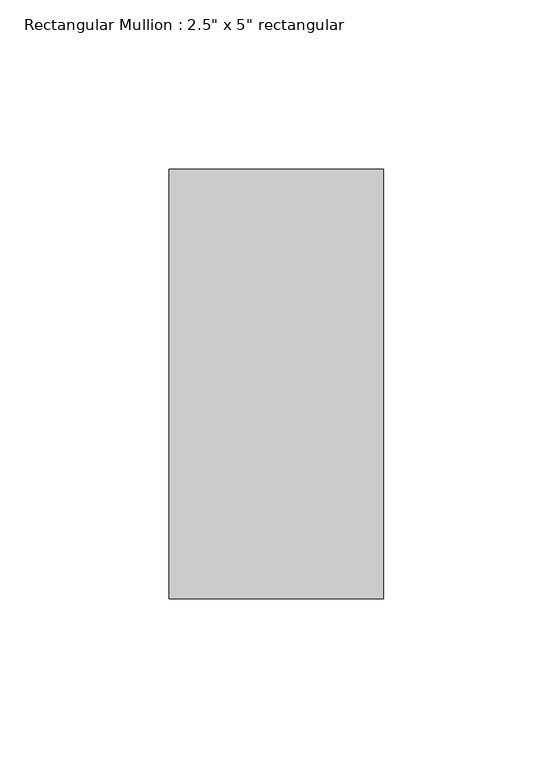
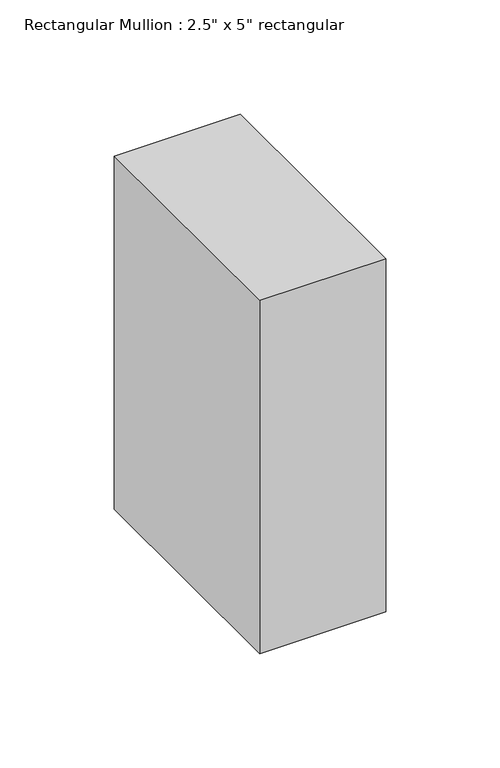
"""IFC4 building model written with IfcOpenShell, lengths in millimetres: member geometry."""

from ifc_helpers import new_model, si_unit, frame, origin, place, context, project, spatial, polyline, outline, extrude, source, transform, mapped, element, save


def member_fa619fab(model_context):
    return source(origin(), model_context, "Body", "SweptSolid", [
        extrude(outline(polyline([(0.0, 63.5), (0.0, -63.5), (-63.5, -63.5), (-63.5, 63.5), (0.0, 63.5)])), frame((0.0, 0.0, -188.3833333), z_axis=(0.0, 0.0, 1.0), x_axis=(1.0, 0.0, 0.0)), (0.0, 0.0, 1.0), 188.3833333),
    ])


if __name__ == "__main__":
    model = new_model("IFC4")
    model_context = context("Model", 3, world=origin())
    ifc_project = project(units=[si_unit("LENGTHUNIT", "METRE", prefix="MILLI")], contexts=[model_context])
    site = spatial("IfcSite", under=ifc_project)
    building = spatial("IfcBuilding", under=site)
    placement = place(None, origin())
    member_shape = member_fa619fab(model_context)
    element("IfcMember", 1, ObjectType="Rectangular Mullion : 2.5\" x 5\" rectangular", at=placement, inside=building, context=model_context, shape_type="MappedRepresentation", body=[
        mapped(member_shape, transform((0.0, 0.0, 0.0), x_axis=(1.0, 0.0, 0.0), y_axis=(0.0, 1.0, 0.0), z_axis=(0.0, 0.0, 1.0))),
    ])
    save(model, "model.ifc")

# Revit data of these elements
# Type "Rectangular Mullion : 2.5\" x 5\" rectangular"
#   built-in parameter 1007304 = 0.416667 (stored number, unit not read)
#   built-in parameter 1007301 = 0.104167 (stored number, unit not read)
#   built-in parameter 1007300 = 0.104167 (stored number, unit not read)
# Element 1 (IfcMember, "Rectangular Mullion : 2.5\" x 5\" rectangular")
#   Materials on its faces: "Aluminum"
# Materials
#   "Aluminum": class "Metal", colour RGB 247 247 247, transparency 0, Description = "Aluminum 6061", Cost = 0
